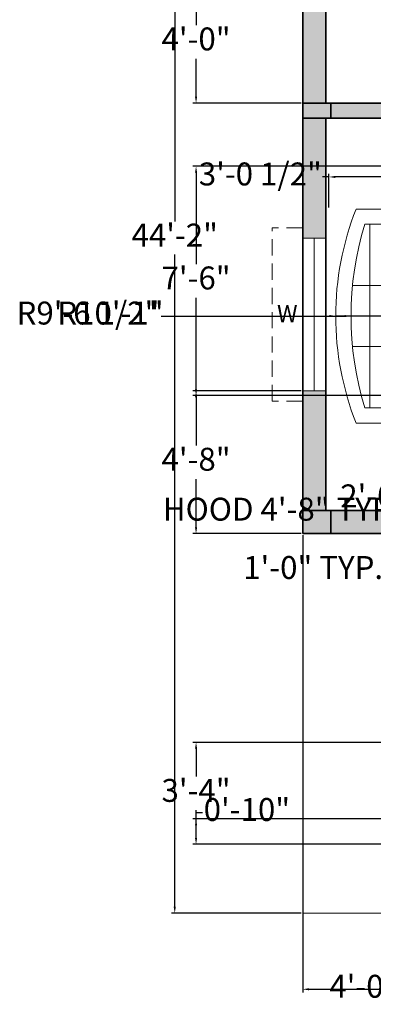
# Model space of a CAD drawing. Units: inches. Extents: x 9689 to 10369, y 10965 to 11626.
# Tile 1 of 11: x 9691 to 9830, y 10973 to 11359. Entities that reach past the tile are written whole.
import ezdxf

# ---------------------------------------------------------------- set-up
doc = ezdxf.new("R2010")
doc.units = ezdxf.units.IN
doc.linetypes.add('DASHED2', pattern=[9.525, 6.35, -3.175])
for name, color, linetype, lineweight in [('A-ANNO-DIMS', 2, 'Continuous', 18), ('A-ANNO-TEXT', 7, 'Continuous', 18), ('A-COLS', 7, 'Continuous', 35), ('A-FURN', 8, 'Continuous', 18), ('A-GLAZ', 4, 'Continuous', 18), ('A-GLAZ-OVHD', 4, 'DASHED2', 13), ('A-WALL', 7, 'Continuous', 35), ('A-WALL-PATT', 252, 'Continuous', 13)]:
    doc.layers.add(name, color=color, linetype=linetype, lineweight=lineweight)
doc.layers.add('A-COLS-PATT', color=18, linetype='Continuous', lineweight=13, true_color=0x000000)
doc.styles.get("Standard").update_dxf_attribs({"font": 'arial.ttf'})
doc.dimstyles.new('ISO-25', dxfattribs={"dimtxt": 9, "dimasz": 2.5, "dimexe": 1.25, "dimexo": 0.625, "dimgap": 2, "dimtad": 0, "dimtih": 1, "dimtoh": 1, "dimdec": 1, "dimlunit": 4, "dimtxsty": 'Standard', "dimcen": 2.5, "dimadec": 0, "dimazin": 0, "dimtfac": 0.5, "dimtdec": 1, "dimtmove": 0, "dimatfit": 3, "dimfxl": 1, "dimarcsym": 0})

# ---------------------------------------------------------------- blocks, each defined once
blk = doc.blocks.new('Sofa - Roundback 7 ft.')
for p, q in [((-12.00002, -32.4421), (-12.00003, -6.5971)), ((11.99997, -32.4421), (11.99998, -6.5971)), ((-36.000027, -34), (-36.000027, -11.4696)), ((35.99998, -34), (35.99998, -11.4696)), ((-35.999844, -13.3819), (35.9998, -13.3819)), ((-36.000027, -32.4421), (35.99998, -32.4421))]:
    blk.add_line(p, q)
for points in [[(-36.000027, -34), (-42.000027, -34), (-42.000027, -8)], [(41.99998, -8), (41.99998, -34), (35.99998, -34)]]:
    blk.add_lwpolyline(points)
for centre, radius, start, end in [((0, -114.25), 114.25, 68.43141, 111.5686), ((-0.00001, -127.1968), 121.1968, 72.72033, 107.2797)]:
    blk.add_arc(centre, radius, start, end)
blk = doc.blocks.new('*D20')
at = {"layer": 'A-ANNO-DIMS', "color": 0, "lineweight": -2, "transparency": 16777216}
for p, q in [((9801.43, 11538.63), (9750.54, 11538.63)), ((9751.79, 11536.13), (9751.79, 11280.15)), ((9751.79, 11011.13), (9751.79, 11267.11)), ((9801.43, 11008.63), (9750.54, 11008.63))]:
    blk.add_line(p, q, dxfattribs=at)
at = {"layer": 'A-ANNO-DIMS', "color": 0, "transparency": 16777216}
for points in [[(9751.38, 11536.13), (9752.21, 11536.13), (9751.79, 11538.63)], [(9751.38, 11011.13), (9752.21, 11011.13), (9751.79, 11008.63)]]:
    blk.add_solid(points, dxfattribs=at)
at = {"layer": 'Defpoints', "color": 0, "transparency": 16777216}
for p in [(9802.06, 11538.63), (9751.79, 11008.63), (9802.06, 11008.63)]:
    blk.add_point(p, dxfattribs=at)
at = {"layer": 'A-ANNO-DIMS', "color": 0, "transparency": 16777216, "insert": (9751.79, 11273.63), "char_height": 9, "attachment_point": 5}
blk.add_mtext('44\'-2"', dxfattribs=at)
blk = doc.blocks.new('WINDOW-HOOD-68')
for p, q in [((12, 68), (0, 68)), ((0, 0), (0, 68)), ((12, 0), (0, 0))]:
    blk.add_line(p, q)
blk = doc.blocks.new('WINDOW-60')
for p, q in [((0, 60), (9, 60)), ((4.5, 60), (4.5, 0)), ((0, 0), (9, 0))]:
    blk.add_line(p, q)
blk = doc.blocks.new('*D38')
at = {"layer": 'A-ANNO-DIMS', "color": 0, "lineweight": -2, "transparency": 16777216}
for p, q in [((9846.06, 11158.26), (9846.06, 11167.28)), ((9902.06, 11158.26), (9902.06, 11167.28)), ((9846.06, 11166.03), (9843.56, 11166.03)), ((9899.56, 11166.03), (9848.56, 11166.03))]:
    blk.add_line(p, q, dxfattribs=at)
at = {"layer": 'A-ANNO-DIMS', "color": 0, "transparency": 16777216}
for points in [[(9848.56, 11166.45), (9848.56, 11165.61), (9846.06, 11166.03)], [(9899.56, 11166.45), (9899.56, 11165.61), (9902.06, 11166.03)]]:
    blk.add_solid(points, dxfattribs=at)
at = {"layer": 'Defpoints', "color": 0, "transparency": 16777216}
for p in [(9846.06, 11166.03), (9846.06, 11157.63), (9902.06, 11157.63)]:
    blk.add_point(p, dxfattribs=at)
at = {"layer": 'A-ANNO-DIMS', "color": 0, "transparency": 16777216, "insert": (9793.76, 11166.03), "char_height": 9, "attachment_point": 5}
blk.add_mtext('HOOD 4\'-8" TYP.', dxfattribs=at)
blk = doc.blocks.new('*D39')
at = {"layer": 'A-ANNO-DIMS', "color": 0, "lineweight": -2, "transparency": 16777216}
for p, q in [((9845.43, 11157.63), (9836.41, 11157.63)), ((9837.66, 11155.13), (9837.66, 11148.13)), ((9845.43, 11145.63), (9836.41, 11145.63)), ((9837.66, 11145.63), (9837.66, 11143.13)), ((9837.66, 11143.13), (9835.16, 11143.13))]:
    blk.add_line(p, q, dxfattribs=at)
at = {"layer": 'A-ANNO-DIMS', "color": 0, "transparency": 16777216}
for points in [[(9837.24, 11155.13), (9838.07, 11155.13), (9837.66, 11157.63)], [(9837.24, 11148.13), (9838.07, 11148.13), (9837.66, 11145.63)]]:
    blk.add_solid(points, dxfattribs=at)
at = {"layer": 'Defpoints', "color": 0, "transparency": 16777216}
for p in [(9846.06, 11157.63), (9837.66, 11145.63), (9846.06, 11145.63)]:
    blk.add_point(p, dxfattribs=at)
at = {"layer": 'A-ANNO-DIMS', "color": 0, "transparency": 16777216, "insert": (9806.15, 11143.13), "char_height": 9, "attachment_point": 5}
blk.add_mtext('1\'-0" TYP.', dxfattribs=at)
blk = doc.blocks.new('*D55')
at = {"layer": 'A-ANNO-DIMS', "color": 0, "lineweight": -2, "transparency": 16777216}
for p, q in [((9812.34, 11285.64), (9812.34, 11298.87)), ((9849.01, 11285.64), (9849.01, 11298.87)), ((9812.34, 11297.62), (9809.84, 11297.62)), ((9846.51, 11297.62), (9814.84, 11297.62))]:
    blk.add_line(p, q, dxfattribs=at)
at = {"layer": 'A-ANNO-DIMS', "color": 0, "transparency": 16777216}
for points in [[(9814.84, 11298.03), (9814.84, 11297.2), (9812.34, 11297.62)], [(9846.51, 11298.03), (9846.51, 11297.2), (9849.01, 11297.62)]]:
    blk.add_solid(points, dxfattribs=at)
at = {"layer": 'Defpoints', "color": 0, "transparency": 16777216}
for p in [(9812.34, 11297.62), (9812.34, 11285.02), (9849.01, 11285.02)]:
    blk.add_point(p, dxfattribs=at)
at = {"layer": 'A-ANNO-DIMS', "color": 0, "transparency": 16777216, "insert": (9785.4, 11297.62), "char_height": 9, "attachment_point": 5}
blk.add_mtext('3\'-0 1/2"', dxfattribs=at)
blk = doc.blocks.new('*D59')
at = {"layer": 'A-ANNO-DIMS', "color": 0, "lineweight": -2, "transparency": 16777216}
for p, q in [((9867.98, 11174.67), (9867.98, 11170)), ((9892.42, 11174.67), (9892.42, 11170)), ((9867.98, 11171.25), (9865.48, 11171.25)), ((9889.92, 11171.25), (9870.48, 11171.25))]:
    blk.add_line(p, q, dxfattribs=at)
at = {"layer": 'A-ANNO-DIMS', "color": 0, "transparency": 16777216}
for points in [[(9870.48, 11171.67), (9870.48, 11170.83), (9867.98, 11171.25)], [(9889.92, 11171.67), (9889.92, 11170.83), (9892.42, 11171.25)]]:
    blk.add_solid(points, dxfattribs=at)
at = {"layer": 'Defpoints', "color": 0, "transparency": 16777216}
for p in [(9867.98, 11175.3), (9892.42, 11175.3), (9867.98, 11171.25)]:
    blk.add_point(p, dxfattribs=at)
at = {"layer": 'A-ANNO-DIMS', "color": 0, "transparency": 16777216, "insert": (9840.96, 11171.25), "char_height": 9, "attachment_point": 5}
blk.add_mtext('2\'-0 1/2"', dxfattribs=at)
blk = doc.blocks.new('*D67')
at = {"layer": 'A-ANNO-DIMS', "color": 0, "lineweight": -2, "transparency": 16777216}
for p, q in [((9802.06, 11157.01), (9802.06, 10977.48)), ((9905.06, 11157.01), (9905.06, 10977.48)), ((9804.56, 10978.73), (9839.59, 10978.73)), ((9902.56, 10978.73), (9867.53, 10978.73))]:
    blk.add_line(p, q, dxfattribs=at)
at = {"layer": 'A-ANNO-DIMS', "color": 0, "transparency": 16777216}
for points in [[(9804.56, 10979.15), (9804.56, 10978.31), (9802.06, 10978.73)], [(9902.56, 10979.15), (9902.56, 10978.31), (9905.06, 10978.73)]]:
    blk.add_solid(points, dxfattribs=at)
at = {"layer": 'Defpoints', "color": 0, "transparency": 16777216}
for p in [(9802.06, 11157.63), (9905.06, 11157.63), (9905.06, 10978.73)]:
    blk.add_point(p, dxfattribs=at)
at = {"layer": 'A-ANNO-DIMS', "color": 0, "transparency": 16777216, "insert": (9853.56, 10978.73), "char_height": 9, "attachment_point": 5}
blk.add_mtext('8\'-7"', dxfattribs=at)
blk = doc.blocks.new('*D68')
at = {"layer": 'A-ANNO-DIMS', "color": 0, "lineweight": -2, "transparency": 16777216}
for p, q in [((9929.43, 11075.63), (9758.91, 11075.63)), ((9760.16, 11073.13), (9760.16, 11062.23)), ((9760.16, 11038.13), (9760.16, 11049.03)), ((9929.43, 11035.63), (9758.91, 11035.63))]:
    blk.add_line(p, q, dxfattribs=at)
at = {"layer": 'A-ANNO-DIMS', "color": 0, "transparency": 16777216}
for points in [[(9759.74, 11073.13), (9760.57, 11073.13), (9760.16, 11075.63)], [(9759.74, 11038.13), (9760.57, 11038.13), (9760.16, 11035.63)]]:
    blk.add_solid(points, dxfattribs=at)
at = {"layer": 'Defpoints', "color": 0, "transparency": 16777216}
for p in [(9760.16, 11075.63), (9930.06, 11075.63), (9930.06, 11035.63)]:
    blk.add_point(p, dxfattribs=at)
at = {"layer": 'A-ANNO-DIMS', "color": 0, "transparency": 16777216, "insert": (9760.16, 11055.63), "char_height": 9, "attachment_point": 5}
blk.add_mtext('3\'-4"', dxfattribs=at)
blk = doc.blocks.new('*D73')
at = {"layer": 'A-ANNO-DIMS', "color": 0, "lineweight": -2, "transparency": 16777216}
for p, q in [((10010.43, 11301.79), (9758.91, 11301.79)), ((9760.16, 11299.29), (9760.16, 11263.38)), ((9760.16, 11214.29), (9760.16, 11250.19)), ((10010.43, 11211.79), (9758.91, 11211.79))]:
    blk.add_line(p, q, dxfattribs=at)
at = {"layer": 'A-ANNO-DIMS', "color": 0, "transparency": 16777216}
for points in [[(9759.74, 11299.29), (9760.57, 11299.29), (9760.16, 11301.79)], [(9759.74, 11214.29), (9760.57, 11214.29), (9760.16, 11211.79)]]:
    blk.add_solid(points, dxfattribs=at)
at = {"layer": 'Defpoints', "color": 0, "transparency": 16777216}
for p in [(9760.16, 11301.79), (10011.06, 11301.79), (10011.06, 11211.79)]:
    blk.add_point(p, dxfattribs=at)
at = {"layer": 'A-ANNO-DIMS', "color": 0, "transparency": 16777216, "insert": (9760.16, 11256.79), "char_height": 9, "attachment_point": 5}
blk.add_mtext('7\'-6"', dxfattribs=at)
blk = doc.blocks.new('*D87')
at = {"layer": 'A-ANNO-DIMS', "color": 0, "lineweight": -2, "transparency": 16777216}
for p, q in [((9802.06, 11157.01), (9802.06, 10977.48)), ((9850.06, 11157.01), (9850.06, 10977.48)), ((9804.56, 10978.73), (9811.91, 10978.73)), ((9847.56, 10978.73), (9840.2, 10978.73))]:
    blk.add_line(p, q, dxfattribs=at)
at = {"layer": 'A-ANNO-DIMS', "color": 0, "transparency": 16777216}
for points in [[(9804.56, 10979.15), (9804.56, 10978.31), (9802.06, 10978.73)], [(9847.56, 10979.15), (9847.56, 10978.31), (9850.06, 10978.73)]]:
    blk.add_solid(points, dxfattribs=at)
at = {"layer": 'Defpoints', "color": 0, "transparency": 16777216}
for p in [(9802.06, 11157.63), (9850.06, 11157.63), (9850.06, 10978.73)]:
    blk.add_point(p, dxfattribs=at)
at = {"layer": 'A-ANNO-DIMS', "color": 0, "transparency": 16777216, "insert": (9826.06, 10978.73), "char_height": 9, "attachment_point": 5}
blk.add_mtext('4\'-0"', dxfattribs=at)
blk = doc.blocks.new('*D90')
at = {"layer": 'A-ANNO-DIMS', "color": 0, "lineweight": -2, "transparency": 16777216}
for p, q in [((9801.43, 11213.63), (9758.91, 11213.63)), ((9760.16, 11211.13), (9760.16, 11192.23)), ((9760.16, 11160.13), (9760.16, 11179.03)), ((9801.43, 11157.63), (9758.91, 11157.63))]:
    blk.add_line(p, q, dxfattribs=at)
at = {"layer": 'A-ANNO-DIMS', "color": 0, "transparency": 16777216}
for points in [[(9759.74, 11211.13), (9760.57, 11211.13), (9760.16, 11213.63)], [(9759.74, 11160.13), (9760.57, 11160.13), (9760.16, 11157.63)]]:
    blk.add_solid(points, dxfattribs=at)
at = {"layer": 'Defpoints', "color": 0, "transparency": 16777216}
for p in [(9760.16, 11213.63), (9802.06, 11213.63), (9802.06, 11157.63)]:
    blk.add_point(p, dxfattribs=at)
at = {"layer": 'A-ANNO-DIMS', "color": 0, "transparency": 16777216, "insert": (9760.16, 11185.63), "char_height": 9, "attachment_point": 5}
blk.add_mtext('4\'-8"', dxfattribs=at)
blk = doc.blocks.new('*D99')
at = {"layer": 'A-ANNO-DIMS', "color": 0, "lineweight": -2, "transparency": 16777216}
for p, q in [((9922.43, 11374.63), (9758.91, 11374.63)), ((9760.16, 11372.13), (9760.16, 11357.23)), ((9760.16, 11329.13), (9760.16, 11344.03)), ((9801.43, 11326.63), (9758.91, 11326.63))]:
    blk.add_line(p, q, dxfattribs=at)
at = {"layer": 'A-ANNO-DIMS', "color": 0, "transparency": 16777216}
for points in [[(9759.74, 11372.13), (9760.57, 11372.13), (9760.16, 11374.63)], [(9759.74, 11329.13), (9760.57, 11329.13), (9760.16, 11326.63)]]:
    blk.add_solid(points, dxfattribs=at)
at = {"layer": 'Defpoints', "color": 0, "transparency": 16777216}
for p in [(9923.06, 11374.63), (9760.16, 11326.63), (9802.06, 11326.63)]:
    blk.add_point(p, dxfattribs=at)
at = {"layer": 'A-ANNO-DIMS', "color": 0, "transparency": 16777216, "insert": (9760.16, 11350.63), "char_height": 9, "attachment_point": 5}
blk.add_mtext('4\'-0"', dxfattribs=at)
blk = doc.blocks.new('*D113')
at = {"layer": 'A-ANNO-DIMS', "color": 0, "lineweight": -2, "transparency": 16777216}
for p, q in [((9760.16, 11045.63), (9760.16, 11048.13)), ((9760.16, 11048.13), (9762.66, 11048.13)), ((9984.43, 11045.63), (9758.91, 11045.63)), ((9760.16, 11038.13), (9760.16, 11043.13)), ((9984.43, 11035.63), (9758.91, 11035.63))]:
    blk.add_line(p, q, dxfattribs=at)
at = {"layer": 'A-ANNO-DIMS', "color": 0, "transparency": 16777216}
for points in [[(9759.74, 11043.13), (9760.57, 11043.13), (9760.16, 11045.63)], [(9759.74, 11038.13), (9760.57, 11038.13), (9760.16, 11035.63)]]:
    blk.add_solid(points, dxfattribs=at)
at = {"layer": 'Defpoints', "color": 0, "transparency": 16777216}
for p in [(9760.16, 11045.63), (9985.06, 11045.63), (9985.06, 11035.63)]:
    blk.add_point(p, dxfattribs=at)
at = {"layer": 'A-ANNO-DIMS', "color": 0, "transparency": 16777216, "insert": (9780.12, 11048.13), "char_height": 9, "attachment_point": 5}
blk.add_mtext('0\'-10"', dxfattribs=at)
blk = doc.blocks.new('*D124')
at = {"layer": 'A-ANNO-DIMS', "color": 0, "lineweight": -2, "transparency": 16777216}
for p, q in [((9746.46, 11243.02), (9812.51, 11243.02)), ((9929.26, 11243.02), (9815.01, 11243.02))]:
    blk.add_line(p, q, dxfattribs=at)
at = {"layer": 'A-ANNO-DIMS', "color": 0, "transparency": 16777216}
blk.add_solid([(9812.51, 11243.43), (9812.51, 11242.6), (9815.01, 11243.02)], dxfattribs=at)
at = {"layer": 'Defpoints', "color": 0, "transparency": 16777216}
for p in [(9815.01, 11243.02), (9929.26, 11243.02)]:
    blk.add_point(p, dxfattribs=at)
at = {"layer": 'A-ANNO-DIMS', "color": 0, "transparency": 16777216, "insert": (9717.71, 11243.02), "char_height": 9, "attachment_point": 5}
blk.add_mtext('R9\'-6 1/2"', dxfattribs=at)
blk = doc.blocks.new('*D125')
at = {"layer": 'A-ANNO-DIMS', "color": 0, "lineweight": -2, "transparency": 16777216}
for p, q in [((9748.29, 11243.02), (9818.51, 11243.02)), ((9942.21, 11243.02), (9821.01, 11243.02))]:
    blk.add_line(p, q, dxfattribs=at)
at = {"layer": 'A-ANNO-DIMS', "color": 0, "transparency": 16777216}
blk.add_solid([(9818.51, 11243.43), (9818.51, 11242.6), (9821.01, 11243.02)], dxfattribs=at)
at = {"layer": 'Defpoints', "color": 0, "transparency": 16777216}
for p in [(9821.01, 11243.02), (9942.21, 11243.02)]:
    blk.add_point(p, dxfattribs=at)
at = {"layer": 'A-ANNO-DIMS', "color": 0, "transparency": 16777216, "insert": (9726.53, 11243.02), "char_height": 9, "attachment_point": 5}
blk.add_mtext('R10\'-1"', dxfattribs=at)

msp = doc.modelspace()

# ---------------------------------------------------------------- hatches: boundary and pattern name
at = {"layer": 'A-COLS-PATT'}
h = msp.add_hatch(color=256, dxfattribs=at)
h.dxf.hatch_style = 1
h.paths.add_polyline_path([(9813.06, 11326.63), (9811.06, 11326.63), (9802.06, 11326.63), (9802.06, 11320.63), (9811.06, 11320.63), (9813.06, 11320.63)])
h = msp.add_hatch(color=256, dxfattribs=at)
h.dxf.hatch_style = 1
h.paths.add_polyline_path([(9813.06, 11166.63), (9811.06, 11166.63), (9802.06, 11166.63), (9802.06, 11157.63), (9813.06, 11157.63)])
at = {"layer": 'A-WALL-PATT'}
h = msp.add_hatch(dxfattribs=at)
h.set_pattern_fill('ANSI33', color=256)
h.paths.add_polyline_path([(9843.06, 11538.63), (9811.06, 11538.63), (9811.06, 11529.63), (9843.06, 11529.63)])
h.paths.add_polyline_path([(9923.06, 11538.63), (9891.06, 11538.63), (9891.06, 11529.63), (9923.06, 11529.63)])
h.paths.add_polyline_path([(9929.06, 11527.63), (9923.06, 11527.63), (9923.06, 11380.63), (9929.06, 11380.63)])
h.paths.add_polyline_path([(9939.06, 11538.63), (9929.06, 11538.63), (9929.06, 11529.63), (9939.06, 11529.63, -0.071068)])
h.paths.add_polyline_path([(10035.06, 11538.63), (10013.06, 11538.63), (10013.06, 11529.63), (10022.06, 11529.63), (10022.06, 11507.38), (10022.06, 11502.38), (10022.06, 11482.38), (10022.06, 11478.38), (10022.06, 11456.13, -0.038405), (10026.06, 11456.13), (10026.06, 11502.38), (10026.06, 11529.63), (10035.06, 11529.63)])
h.paths.add_polyline_path([(10068.06, 11538.63), (10059.06, 11538.63), (10059.06, 11529.63), (10068.06, 11529.63)])
h.paths.add_polyline_path([(10074.06, 11527.63), (10068.06, 11527.63), (10068.06, 11431.13), (10026.06, 11431.13), (10022.06, 11431.13), (9980.06, 11431.13), (9976.06, 11431.13), (9976.06, 11425.13), (10068.06, 11425.13), (10068.06, 11380.63), (10074.06, 11380.63)])
h.paths.add_polyline_path([(10124.56, 11538.63), (10074.06, 11538.63), (10074.06, 11529.63), (10124.56, 11529.63)])
h.paths.add_polyline_path([(9980.06, 11507.38), (9980.06, 11529.63), (9989.06, 11529.63), (9989.06, 11538.63), (9976.06, 11538.63), (9976.06, 11529.63), (9976.06, 11503.38), (9976.06, 11483.38), (9976.06, 11478.38), (9980.06, 11478.38), (9997.06, 11478.38, -0.038405), (9997.06, 11482.38), (9980.06, 11482.38)])
h.paths.add_polyline_path([(10235.06, 11538.63), (10184.56, 11538.63), (10184.56, 11529.63), (10235.06, 11529.63)])
h.paths.add_polyline_path([(10244.06, 11527.63), (10235.06, 11527.63), (10235.06, 11485.13), (10244.06, 11485.13)])
h.paths.add_polyline_path([(10244.06, 11425.13), (10235.06, 11425.13), (10235.06, 11380.63), (10244.06, 11380.63)])
h.paths.add_polyline_path([(10233.06, 11380.63), (10120.06, 11380.63, -0.038405), (10120.06, 11374.63), (10133.04, 11374.63), (10133.04, 11326.63), (10120.06, 11326.63, -0.038405), (10120.06, 11320.63), (10149.19, 11320.63), (10149.19, 11326.63), (10136.04, 11326.63), (10136.04, 11374.63), (10233.06, 11374.63)])
h.paths.add_polyline_path([(10084.06, 11380.63), (10076.06, 11380.63), (10076.06, 11374.63), (10084.06, 11374.63)])
h.paths.add_polyline_path([(10244.06, 11374.63), (10235.06, 11374.63), (10235.06, 11362.63), (10244.06, 11362.63)])
h.paths.add_polyline_path([(10244.06, 11338.63), (10235.06, 11338.63), (10235.06, 11326.63), (10244.06, 11326.63)])
h.paths.add_polyline_path([(10233.06, 11326.63), (10173.19, 11326.63, -0.055385), (10173.19, 11320.63), (10233.06, 11320.63)], flags=0)
h.paths.add_polyline_path([(10244.06, 11320.63), (10235.06, 11320.63), (10235.06, 11273.63), (10244.06, 11273.63)])
h = msp.add_hatch(dxfattribs=at)
h.set_pattern_fill('ANSI36', color=256)
h.paths.add_polyline_path([(10233.06, 11326.63), (10173.19, 11326.63, -0.055385), (10173.19, 11320.63), (10233.06, 11320.63)])
h.paths.add_polyline_path([(10244.06, 11213.63), (10235.06, 11213.63), (10235.06, 11166.63), (10244.06, 11166.63)])
h.paths.add_polyline_path([(10233.06, 11166.63), (10184.56, 11166.63), (10184.56, 11157.63), (10233.06, 11157.63)])
h.paths.add_polyline_path([(10124.56, 11166.63), (10074.06, 11166.63), (10074.06, 11157.63), (10124.56, 11157.63)])
h.paths.add_polyline_path([(10074.06, 11318.63), (10068.06, 11318.63), (10068.06, 11168.63), (10074.06, 11168.63)])
h.paths.add_polyline_path([(10068.06, 11166.63), (10011.06, 11166.63), (10011.06, 11157.63), (10068.06, 11157.63)])
h.paths.add_polyline_path([(10011.06, 11318.63), (10005.06, 11318.63), (10005.06, 11168.63), (10011.06, 11168.63)])
h.paths.add_polyline_path([(10005.06, 11166.63), (9985.06, 11166.63), (9985.06, 11157.63), (10005.06, 11157.63)])
h.paths.add_polyline_path([(9937.06, 11166.63), (9898.06, 11166.63), (9898.06, 11157.63), (9937.06, 11157.63, -0.042779)])
h.paths.add_polyline_path([(9850.06, 11166.63), (9813.06, 11166.63), (9813.06, 11157.63), (9850.06, 11157.63)])
h.paths.add_polyline_path([(9811.06, 11213.63), (9802.06, 11213.63), (9802.06, 11166.63), (9811.06, 11166.63)])
h.paths.add_polyline_path([(9811.06, 11320.63), (9802.06, 11320.63), (9802.06, 11273.63), (9811.06, 11273.63)])
h.paths.add_polyline_path([(9811.06, 11439.11), (9802.06, 11439.11), (9802.06, 11326.63), (9811.06, 11326.63)])
h.paths.add_polyline_path([(9957.06, 11326.63), (9813.06, 11326.63), (9813.06, 11320.63), (9957.06, 11320.63)])
h.paths.add_polyline_path([(9811.06, 11527.63), (9802.06, 11527.63), (9802.06, 11499.11), (9811.06, 11499.11)])

# ---------------------------------------------------------------- linework, layer by layer
at = {"layer": 'A-ANNO-DIMS'}
msp.add_line((9904.55, 11008.63), (9802.06, 11008.63), dxfattribs=at)
at = {"layer": 'A-COLS'}
for p, q in [((9811.06, 11326.63), (9802.06, 11326.63)), ((9813.06, 11326.63), (9813.06, 11320.63)), ((9811.06, 11320.63), (9802.06, 11320.63)), ((9811.06, 11166.63), (9802.06, 11166.63)), ((9813.06, 11166.63), (9813.06, 11157.63))]:
    msp.add_line(p, q, dxfattribs=at)
at = {"layer": 'A-WALL'}
for p, q in [((9802.06, 11157.63), (9802.06, 11538.63)), ((9811.06, 11326.63), (9811.06, 11529.63)), ((9811.06, 11326.63), (9923.06, 11326.63)), ((9811.06, 11326.63), (9957.06, 11326.63)), ((9811.06, 11166.63), (9811.06, 11320.63)), ((9811.06, 11320.63), (9957.06, 11320.63)), ((9937.06, 11166.63), (9811.06, 11166.63)), ((9937.06, 11157.63), (9802.06, 11157.63))]:
    msp.add_line(p, q, dxfattribs=at)

# ---------------------------------------------------------------- block references
at = {"layer": 'A-FURN', "rotation": 89.99997936313842}
msp.add_blockref('Sofa - Roundback 7 ft.', (9815.01, 11243.02), dxfattribs=at)
at = {"layer": 'A-GLAZ'}
msp.add_blockref('WINDOW-60', (9802.06, 11213.63), dxfattribs=at)
at = {"layer": 'A-GLAZ-OVHD'}
msp.add_blockref('WINDOW-HOOD-68', (9790.06, 11209.63), dxfattribs=at)

# ---------------------------------------------------------------- texts
at = {"layer": 'A-ANNO-TEXT', "insert": (9791.96, 11247.31), "char_height": 6.729, "attachment_point": 1}
msp.add_mtext_dynamic_manual_height_columns('{\\fArial|b1|i0|c0|p34;W}', width=31.3623, gutter_width=33.65, heights=[0], dxfattribs=at)

# ---------------------------------------------------------------- dimensions: what is measured, and where the dimension line sits
at = {"layer": 'A-ANNO-DIMS'}
for base, p1, p2, angle, override, picture, middle in [((9751.79, 11008.63), (9802.06, 11538.63), (9802.06, 11008.63), 90, {"dimclrd": 0, "dimclre": 0, "dimclrt": 0}, '*D20', (9751.79, 11273.63)), ((9760.16, 11326.63), (9923.06, 11374.63), (9802.06, 11326.63), 90, {"dimdec": 1, "dimlfac": 1, "dimrnd": 0, "dimzin": 1, "dimdsep": 46, "dimlunit": 4, "dimfrac": 2}, '*D99', (9760.16, 11350.63)), ((9812.34, 11297.62), (9849.01, 11285.02), (9812.34, 11285.02), 180, {"dimdec": 1, "dimlfac": 1, "dimrnd": 0, "dimzin": 1, "dimdsep": 46, "dimlunit": 4, "dimfrac": 2}, '*D55', (9785.4, 11297.62)), ((9760.16, 11301.79), (10011.06, 11211.79), (10011.06, 11301.79), 90, {"dimdec": 1, "dimlfac": 1, "dimrnd": 0, "dimzin": 1, "dimdsep": 46, "dimlunit": 4, "dimfrac": 2}, '*D73', (9760.16, 11256.79)), ((9760.16, 11213.63), (9802.06, 11157.63), (9802.06, 11213.63), 90, {"dimdec": 1, "dimlfac": 1, "dimrnd": 0, "dimzin": 1, "dimdsep": 46, "dimlunit": 4, "dimfrac": 2}, '*D90', (9760.16, 11185.63)), ((9867.98, 11171.25), (9892.42, 11175.3), (9867.98, 11175.3), 180, {"dimdec": 1, "dimlfac": 1, "dimrnd": 0, "dimzin": 1, "dimdsep": 46, "dimlunit": 4, "dimfrac": 2}, '*D59', (9840.96, 11171.25)), ((9760.16, 11075.63), (9930.06, 11035.63), (9930.06, 11075.63), 90, {"dimdec": 1, "dimlfac": 1, "dimrnd": 0, "dimzin": 1, "dimdsep": 46, "dimlunit": 4, "dimfrac": 2}, '*D68', (9760.16, 11055.63)), ((9760.16, 11045.63), (9985.06, 11035.63), (9985.06, 11045.63), 90, {"dimdec": 1, "dimlfac": 1, "dimrnd": 0, "dimzin": 1, "dimdsep": 46, "dimlunit": 4, "dimfrac": 2}, '*D113', (9780.12, 11048.13))]:
    dim = msp.add_linear_dim(base=base, p1=p1, p2=p2, angle=angle, dimstyle='ISO-25', override=override, dxfattribs=at)
    dim.commit()
    dim.dimension.update_dxf_attribs({"geometry": picture, "text_midpoint": middle})
for center, mpoint, picture, middle in [((9929.26068, 11243.017795), (9815.01068, 11243.018), '*D124', (9746.46068, 11243.018123)), ((9942.21, 11243.02), (9821.01, 11243.02), '*D125', (9748.29, 11243.02))]:
    dim = msp.add_radius_dim(center=center, mpoint=mpoint, dimstyle='ISO-25', override={"dimdec": 1, "dimlfac": 1, "dimrnd": 0, "dimzin": 1, "dimdsep": 46, "dimlunit": 4, "dimfrac": 2}, dxfattribs=at)
    dim.commit()
    dim.dimension.update_dxf_attribs({"geometry": picture, "text_midpoint": middle, "dimtype": 164})
for base, p1, p2, angle, text, picture, middle in [((9846.06, 11166.03), (9902.06, 11157.63), (9846.06, 11157.63), 180, 'HOOD <> TYP.', '*D38', (9793.76, 11166.03)), ((9837.66, 11145.63), (9846.06, 11157.63), (9846.06, 11145.63), 270, '<> TYP.', '*D39', (9806.15, 11143.13))]:
    dim = msp.add_linear_dim(base=base, p1=p1, p2=p2, angle=angle, text=text, dimstyle='ISO-25', override={"dimdec": 1, "dimlfac": 1, "dimrnd": 0, "dimzin": 1, "dimdsep": 46, "dimlunit": 4, "dimfrac": 2}, dxfattribs=at)
    dim.commit()
    dim.dimension.update_dxf_attribs({"geometry": picture, "text_midpoint": middle})
for base, p2, picture, middle in [((9905.06, 10978.73), (9905.06, 11157.63), '*D67', (9853.56, 10978.73)), ((9850.06, 10978.73), (9850.06, 11157.63), '*D87', (9826.06, 10978.73))]:
    dim = msp.add_linear_dim(base=base, p1=(9802.06, 11157.63), p2=p2, dimstyle='ISO-25', override={"dimdec": 1, "dimlfac": 1, "dimrnd": 0, "dimzin": 1, "dimdsep": 46, "dimlunit": 4, "dimfrac": 2}, dxfattribs=at)
    dim.commit()
    dim.dimension.update_dxf_attribs({"geometry": picture, "text_midpoint": middle})

doc.saveas('drawing.dxf')
